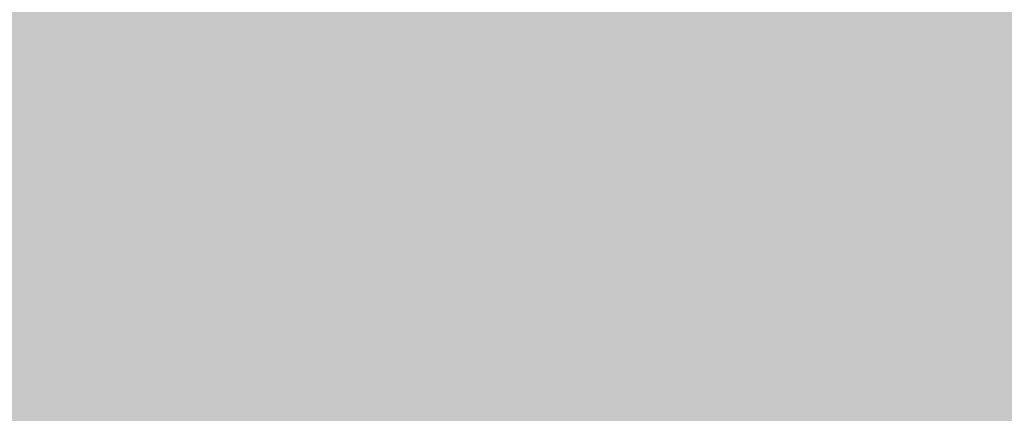
# Model space of a CAD drawing. Units: millimetres. Extents: x -22994 to 29398, y -19990 to 20176.
# Tile 100 of 135: x 229.428 to 230.597, y 84.732 to 85.199. Entities that reach past the tile are written whole.
import ezdxf
from ezdxf import colors
from ezdxf.entities.mleader import LeaderData, LeaderLine
from ezdxf.math import Vec2, Vec3

# ---------------------------------------------------------------- set-up
doc = ezdxf.new("R2010")
doc.units = ezdxf.units.MM
doc.header["$MEASUREMENT"] = 0
doc.layers.add('M-ANNO-TEXT', color=7, linetype='Continuous', lineweight=25)
doc.layers.add('M-DIMS', color=2, linetype='Continuous', lineweight=18)
doc.styles.get("Standard").update_dxf_attribs({"font": 'arial.ttf'})
doc.dimstyles.get("Standard").update_dxf_attribs({"dimtxt": 0.18, "dimasz": 10000, "dimexe": 0.18, "dimexo": 0.0625, "dimgap": 0.09, "dimtad": 0, "dimtih": 1, "dimtoh": 1, "dimdec": 0, "dimzin": 0, "dimdsep": 46, "dimtxsty": 'Standard', "dimcen": 0.09, "dimadec": 0, "dimazin": 0, "dimtfac": 1, "dimtdec": 0, "dimtofl": 0, "dimtmove": 0, "dimatfit": 3, "dimfxl": 1, "dimtolj": 1, "dimtzin": 0, "dimlwd": 30, "dimarcsym": 0})

# ---------------------------------------------------------------- blocks, each defined once
blk = doc.blocks.new('*D2')
at = {"layer": 'Defpoints', "color": 0, "transparency": 16777216}
for p in [(6.6773, 10.2713), (290.852, 10.2713), (290.852, -5.0787)]:
    blk.add_point(p, dxfattribs=at)
at = {"layer": 'M-DIMS', "color": 0, "lineweight": -2, "transparency": 16777216}
for p, q in [((6.6773, 10.2088), (6.6773, -5.2587)), ((290.852, 10.2088), (290.852, -5.2587))]:
    blk.add_line(p, q, dxfattribs=at)
at = {"layer": 'M-DIMS', "color": 0, "lineweight": 30, "transparency": 16777216}
for p, q in [((-9993.3227, -5.0787), (-19993.3227, -5.0787)), ((10290.852, -5.0787), (20290.852, -5.0787))]:
    blk.add_line(p, q, dxfattribs=at)
at = {"layer": 'M-DIMS', "color": 0, "transparency": 16777216}
for points in [[(-9993.3227, 1661.5879), (-9993.3227, -1671.7454), (6.6773, -5.0787)], [(10290.852, 1661.5879), (10290.852, -1671.7454), (290.852, -5.0787)]]:
    blk.add_solid(points, dxfattribs=at)
at = {"layer": 'M-DIMS', "color": 0, "transparency": 16777216, "insert": (148.7647, -5.0787), "char_height": 0.18, "attachment_point": 5}
blk.add_mtext('\\A1;284.2', dxfattribs=at)
blk = doc.blocks.new('*D3')
at = {"layer": 'Defpoints', "color": 0, "transparency": 16777216}
for p in [(110.2647, 204.1654), (110.2647, 176.3662), (95.8327, 127.967)]:
    blk.add_point(p, dxfattribs=at)
at = {"layer": 'M-DIMS', "color": 0, "lineweight": -2, "transparency": 16777216}
for p, q in [((95.8327, 128.0295), (95.8327, 204.3454)), ((110.2647, 176.4287), (110.2647, 204.3454))]:
    blk.add_line(p, q, dxfattribs=at)
at = {"layer": 'M-DIMS', "color": 0, "lineweight": 30, "transparency": 16777216}
for p, q in [((-9904.1673, 204.1654), (-19904.1673, 204.1654)), ((10110.2647, 204.1654), (20110.2647, 204.1654))]:
    blk.add_line(p, q, dxfattribs=at)
at = {"layer": 'M-DIMS', "color": 0, "transparency": 16777216}
for points in [[(-9904.1673, 1870.8321), (-9904.1673, -1462.5013), (95.8327, 204.1654)], [(10110.2647, 1870.8321), (10110.2647, -1462.5013), (110.2647, 204.1654)]]:
    blk.add_solid(points, dxfattribs=at)
at = {"layer": 'M-DIMS', "color": 0, "transparency": 16777216, "insert": (103.0487, 204.1654), "char_height": 0.18, "attachment_point": 5}
blk.add_mtext('\\A1;14.432', dxfattribs=at)
blk = doc.blocks.new('*D4')
at = {"layer": 'Defpoints', "color": 0, "transparency": 16777216}
for p in [(116.2647, 204.1654), (110.2647, 176.3662), (116.2647, 176.3662)]:
    blk.add_point(p, dxfattribs=at)
at = {"layer": 'M-DIMS', "color": 0, "lineweight": -2, "transparency": 16777216}
for p, q in [((110.2647, 176.4287), (110.2647, 204.3454)), ((116.2647, 176.4287), (116.2647, 204.3454))]:
    blk.add_line(p, q, dxfattribs=at)
at = {"layer": 'M-DIMS', "color": 0, "lineweight": 30, "transparency": 16777216}
for p, q in [((-9889.7353, 204.1654), (-19889.7353, 204.1654)), ((10116.2647, 204.1654), (20116.2647, 204.1654))]:
    blk.add_line(p, q, dxfattribs=at)
at = {"layer": 'M-DIMS', "color": 0, "transparency": 16777216}
for points in [[(-9889.7353, 1870.8321), (-9889.7353, -1462.5013), (110.2647, 204.1654)], [(10116.2647, 1870.8321), (10116.2647, -1462.5013), (116.2647, 204.1654)]]:
    blk.add_solid(points, dxfattribs=at)
at = {"layer": 'M-DIMS', "color": 0, "transparency": 16777216, "insert": (113.2647, 204.1654), "char_height": 0.18, "attachment_point": 5}
blk.add_mtext('\\A1;6', dxfattribs=at)
blk = doc.blocks.new('*D5')
at = {"layer": 'Defpoints', "color": 0, "transparency": 16777216}
for p in [(181.2647, 204.1654), (116.2647, 176.3662), (181.2647, 176.3662)]:
    blk.add_point(p, dxfattribs=at)
at = {"layer": 'M-DIMS', "color": 0, "lineweight": -2, "transparency": 16777216}
for p, q in [((116.2647, 176.4287), (116.2647, 204.3454)), ((181.2647, 176.4287), (181.2647, 204.3454))]:
    blk.add_line(p, q, dxfattribs=at)
at = {"layer": 'M-DIMS', "color": 0, "lineweight": 30, "transparency": 16777216}
for p, q in [((-9883.7353, 204.1654), (-19883.7353, 204.1654)), ((10181.2647, 204.1654), (20181.2647, 204.1654))]:
    blk.add_line(p, q, dxfattribs=at)
at = {"layer": 'M-DIMS', "color": 0, "transparency": 16777216}
for points in [[(-9883.7353, 1870.8321), (-9883.7353, -1462.5013), (116.2647, 204.1654)], [(10181.2647, 1870.8321), (10181.2647, -1462.5013), (181.2647, 204.1654)]]:
    blk.add_solid(points, dxfattribs=at)
at = {"layer": 'M-DIMS', "color": 0, "transparency": 16777216, "insert": (148.7647, 204.1654), "char_height": 0.18, "attachment_point": 5}
blk.add_mtext('\\A1;65', dxfattribs=at)
blk = doc.blocks.new('*D6')
at = {"layer": 'Defpoints', "color": 0, "transparency": 16777216}
for p in [(187.2647, 204.1654), (181.2647, 176.3662), (187.2647, 176.3662)]:
    blk.add_point(p, dxfattribs=at)
at = {"layer": 'M-DIMS', "color": 0, "lineweight": -2, "transparency": 16777216}
for p, q in [((181.2647, 176.4287), (181.2647, 204.3454)), ((187.2647, 176.4287), (187.2647, 204.3454))]:
    blk.add_line(p, q, dxfattribs=at)
at = {"layer": 'M-DIMS', "color": 0, "lineweight": 30, "transparency": 16777216}
for p, q in [((-9818.7353, 204.1654), (-19818.7353, 204.1654)), ((10187.2647, 204.1654), (20187.2647, 204.1654))]:
    blk.add_line(p, q, dxfattribs=at)
at = {"layer": 'M-DIMS', "color": 0, "transparency": 16777216}
for points in [[(-9818.7353, 1870.8321), (-9818.7353, -1462.5013), (181.2647, 204.1654)], [(10187.2647, 1870.8321), (10187.2647, -1462.5013), (187.2647, 204.1654)]]:
    blk.add_solid(points, dxfattribs=at)
at = {"layer": 'M-DIMS', "color": 0, "transparency": 16777216, "insert": (184.2647, 204.1654), "char_height": 0.18, "attachment_point": 5}
blk.add_mtext('\\A1;6', dxfattribs=at)
blk = doc.blocks.new('*D7')
at = {"layer": 'Defpoints', "color": 0, "transparency": 16777216}
for p in [(201.6967, 204.1654), (187.2647, 176.3662), (201.6967, 127.967)]:
    blk.add_point(p, dxfattribs=at)
at = {"layer": 'M-DIMS', "color": 0, "lineweight": -2, "transparency": 16777216}
for p, q in [((187.2647, 176.4287), (187.2647, 204.3454)), ((201.6967, 128.0295), (201.6967, 204.3454))]:
    blk.add_line(p, q, dxfattribs=at)
at = {"layer": 'M-DIMS', "color": 0, "lineweight": 30, "transparency": 16777216}
for p, q in [((-9812.7353, 204.1654), (-19812.7353, 204.1654)), ((10201.6967, 204.1654), (20201.6967, 204.1654))]:
    blk.add_line(p, q, dxfattribs=at)
at = {"layer": 'M-DIMS', "color": 0, "transparency": 16777216}
for points in [[(-9812.7353, 1870.8321), (-9812.7353, -1462.5013), (187.2647, 204.1654)], [(10201.6967, 1870.8321), (10201.6967, -1462.5013), (201.6967, 204.1654)]]:
    blk.add_solid(points, dxfattribs=at)
at = {"layer": 'M-DIMS', "color": 0, "transparency": 16777216, "insert": (194.4807, 204.1654), "char_height": 0.18, "attachment_point": 5}
blk.add_mtext('\\A1;14.432', dxfattribs=at)
blk = doc.blocks.new('*D8')
at = {"layer": 'Defpoints', "color": 0, "transparency": 16777216}
for p in [(227.6485, 204.1654), (227.6485, 146.7296), (201.6967, 127.967)]:
    blk.add_point(p, dxfattribs=at)
at = {"layer": 'M-DIMS', "color": 0, "lineweight": -2, "transparency": 16777216}
for p, q in [((201.6967, 128.0295), (201.6967, 204.3454)), ((227.6485, 146.7921), (227.6485, 204.3454))]:
    blk.add_line(p, q, dxfattribs=at)
at = {"layer": 'M-DIMS', "color": 0, "lineweight": 30, "transparency": 16777216}
for p, q in [((-9798.3033, 204.1654), (-19798.3033, 204.1654)), ((10227.6485, 204.1654), (20227.6485, 204.1654))]:
    blk.add_line(p, q, dxfattribs=at)
at = {"layer": 'M-DIMS', "color": 0, "transparency": 16777216}
for points in [[(-9798.3033, 1870.8321), (-9798.3033, -1462.5013), (201.6967, 204.1654)], [(10227.6485, 1870.8321), (10227.6485, -1462.5013), (227.6485, 204.1654)]]:
    blk.add_solid(points, dxfattribs=at)
at = {"layer": 'M-DIMS', "color": 0, "transparency": 16777216, "insert": (214.6726, 204.1654), "char_height": 0.18, "attachment_point": 5}
blk.add_mtext('\\A1;25.95', dxfattribs=at)
blk = doc.blocks.new('*D9')
at = {"layer": 'Defpoints', "color": 0, "transparency": 16777216}
for p in [(187.2647, 176.3662), (306.202, 176.3662), (290.852, 10.2713)]:
    blk.add_point(p, dxfattribs=at)
at = {"layer": 'M-DIMS', "color": 0, "lineweight": 30, "transparency": 16777216}
for p, q in [((306.202, 10176.3662), (306.202, 20176.3662)), ((306.202, -9989.7287), (306.202, -19989.7287))]:
    blk.add_line(p, q, dxfattribs=at)
at = {"layer": 'M-DIMS', "color": 0, "lineweight": -2, "transparency": 16777216}
for p, q in [((187.3272, 176.3662), (306.382, 176.3662)), ((290.9145, 10.2713), (306.382, 10.2713))]:
    blk.add_line(p, q, dxfattribs=at)
at = {"layer": 'M-DIMS', "color": 0, "transparency": 16777216}
for points in [[(-1360.4646, 10176.3662), (1972.8687, 10176.3662), (306.202, 176.3662)], [(-1360.4646, -9989.7287), (1972.8687, -9989.7287), (306.202, 10.2713)]]:
    blk.add_solid(points, dxfattribs=at)
at = {"layer": 'M-DIMS', "color": 0, "transparency": 16777216, "insert": (306.202, 93.3187), "char_height": 0.18, "attachment_point": 5}
blk.add_mtext('\\A1;166.1', dxfattribs=at)
blk = doc.blocks.new('*D10')
at = {"layer": 'Defpoints', "color": 0, "transparency": 16777216}
for p in [(125.6498, 136.0713), (133.3459, 136.0713), (133.3459, -5.0787)]:
    blk.add_point(p, dxfattribs=at)
at = {"layer": 'M-DIMS', "color": 0, "lineweight": -2, "transparency": 16777216}
for p, q in [((125.6498, 136.0088), (125.6498, -5.2587)), ((133.3459, 136.0088), (133.3459, -5.2587))]:
    blk.add_line(p, q, dxfattribs=at)
at = {"layer": 'M-DIMS', "color": 0, "lineweight": 30, "transparency": 16777216}
for p, q in [((-9874.3502, -5.0787), (-19874.3502, -5.0787)), ((10133.3459, -5.0787), (20133.3459, -5.0787))]:
    blk.add_line(p, q, dxfattribs=at)
at = {"layer": 'M-DIMS', "color": 0, "transparency": 16777216}
for points in [[(-9874.3502, 1661.5879), (-9874.3502, -1671.7454), (125.6498, -5.0787)], [(10133.3459, 1661.5879), (10133.3459, -1671.7454), (133.3459, -5.0787)]]:
    blk.add_solid(points, dxfattribs=at)
at = {"layer": 'M-DIMS', "color": 0, "transparency": 16777216, "insert": (129.4978, -5.0787), "char_height": 0.18, "attachment_point": 5}
blk.add_mtext('\\A1;7.696', dxfattribs=at)
blk = doc.blocks.new('*D11')
at = {"layer": 'Defpoints', "color": 0, "transparency": 16777216}
for p in [(133.3459, 136.0713), (135.6498, 136.0713), (135.6498, -5.0787)]:
    blk.add_point(p, dxfattribs=at)
at = {"layer": 'M-DIMS', "color": 0, "lineweight": -2, "transparency": 16777216}
for p, q in [((133.3459, 136.0088), (133.3459, -5.2587)), ((135.6498, 136.0088), (135.6498, -5.2587))]:
    blk.add_line(p, q, dxfattribs=at)
at = {"layer": 'M-DIMS', "color": 0, "lineweight": 30, "transparency": 16777216}
for p, q in [((-9866.6541, -5.0787), (-19866.6541, -5.0787)), ((10135.6498, -5.0787), (20135.6498, -5.0787))]:
    blk.add_line(p, q, dxfattribs=at)
at = {"layer": 'M-DIMS', "color": 0, "transparency": 16777216}
for points in [[(-9866.6541, 1661.5879), (-9866.6541, -1671.7454), (133.3459, -5.0787)], [(10135.6498, 1661.5879), (10135.6498, -1671.7454), (135.6498, -5.0787)]]:
    blk.add_solid(points, dxfattribs=at)
at = {"layer": 'M-DIMS', "color": 0, "transparency": 16777216, "insert": (134.4978, -5.0787), "char_height": 0.18, "attachment_point": 5}
blk.add_mtext('\\A1;2.304', dxfattribs=at)
blk = doc.blocks.new('*D12')
at = {"layer": 'Defpoints', "color": 0, "transparency": 16777216}
for p in [(135.6498, 136.0713), (145.6498, 136.0713), (145.6498, -5.0787)]:
    blk.add_point(p, dxfattribs=at)
at = {"layer": 'M-DIMS', "color": 0, "lineweight": -2, "transparency": 16777216}
for p, q in [((135.6498, 136.0088), (135.6498, -5.2587)), ((145.6498, 136.0088), (145.6498, -5.2587))]:
    blk.add_line(p, q, dxfattribs=at)
at = {"layer": 'M-DIMS', "color": 0, "lineweight": 30, "transparency": 16777216}
for p, q in [((-9864.3502, -5.0787), (-19864.3502, -5.0787)), ((10145.6498, -5.0787), (20145.6498, -5.0787))]:
    blk.add_line(p, q, dxfattribs=at)
at = {"layer": 'M-DIMS', "color": 0, "transparency": 16777216}
for points in [[(-9864.3502, 1661.5879), (-9864.3502, -1671.7454), (135.6498, -5.0787)], [(10145.6498, 1661.5879), (10145.6498, -1671.7454), (145.6498, -5.0787)]]:
    blk.add_solid(points, dxfattribs=at)
at = {"layer": 'M-DIMS', "color": 0, "transparency": 16777216, "insert": (140.6498, -5.0787), "char_height": 0.18, "attachment_point": 5}
blk.add_mtext('\\A1;10', dxfattribs=at)
blk = doc.blocks.new('*D13')
at = {"layer": 'Defpoints', "color": 0, "transparency": 16777216}
for p in [(145.6498, 136.0713), (155.6498, 136.0713), (155.6498, -5.0787)]:
    blk.add_point(p, dxfattribs=at)
at = {"layer": 'M-DIMS', "color": 0, "lineweight": -2, "transparency": 16777216}
for p, q in [((145.6498, 136.0088), (145.6498, -5.2587)), ((155.6498, 136.0088), (155.6498, -5.2587))]:
    blk.add_line(p, q, dxfattribs=at)
at = {"layer": 'M-DIMS', "color": 0, "lineweight": 30, "transparency": 16777216}
for p, q in [((-9854.3502, -5.0787), (-19854.3502, -5.0787)), ((10155.6498, -5.0787), (20155.6498, -5.0787))]:
    blk.add_line(p, q, dxfattribs=at)
at = {"layer": 'M-DIMS', "color": 0, "transparency": 16777216}
for points in [[(-9854.3502, 1661.5879), (-9854.3502, -1671.7454), (145.6498, -5.0787)], [(10155.6498, 1661.5879), (10155.6498, -1671.7454), (155.6498, -5.0787)]]:
    blk.add_solid(points, dxfattribs=at)
at = {"layer": 'M-DIMS', "color": 0, "transparency": 16777216, "insert": (150.6498, -5.0787), "char_height": 0.18, "attachment_point": 5}
blk.add_mtext('\\A1;10', dxfattribs=at)
blk = doc.blocks.new('*D14')
at = {"layer": 'Defpoints', "color": 0, "transparency": 16777216}
for p in [(155.6498, 136.0713), (165.6498, 136.0713), (165.6498, -5.0787)]:
    blk.add_point(p, dxfattribs=at)
at = {"layer": 'M-DIMS', "color": 0, "lineweight": -2, "transparency": 16777216}
for p, q in [((155.6498, 136.0088), (155.6498, -5.2587)), ((165.6498, 136.0088), (165.6498, -5.2587))]:
    blk.add_line(p, q, dxfattribs=at)
at = {"layer": 'M-DIMS', "color": 0, "lineweight": 30, "transparency": 16777216}
for p, q in [((-9844.3502, -5.0787), (-19844.3502, -5.0787)), ((10165.6498, -5.0787), (20165.6498, -5.0787))]:
    blk.add_line(p, q, dxfattribs=at)
at = {"layer": 'M-DIMS', "color": 0, "transparency": 16777216}
for points in [[(-9844.3502, 1661.5879), (-9844.3502, -1671.7454), (155.6498, -5.0787)], [(10165.6498, 1661.5879), (10165.6498, -1671.7454), (165.6498, -5.0787)]]:
    blk.add_solid(points, dxfattribs=at)
at = {"layer": 'M-DIMS', "color": 0, "transparency": 16777216, "insert": (160.6498, -5.0787), "char_height": 0.18, "attachment_point": 5}
blk.add_mtext('\\A1;10', dxfattribs=at)
blk = doc.blocks.new('*D15')
at = {"layer": 'Defpoints', "color": 0, "transparency": 16777216}
for p in [(173.3459, 154.788), (173.3459, 136.0713), (306.202, 136.0713)]:
    blk.add_point(p, dxfattribs=at)
at = {"layer": 'M-DIMS', "color": 0, "lineweight": 30, "transparency": 16777216}
for p, q in [((306.202, 10154.788), (306.202, 20154.788)), ((306.202, -9863.9287), (306.202, -19863.9287))]:
    blk.add_line(p, q, dxfattribs=at)
at = {"layer": 'M-DIMS', "color": 0, "lineweight": -2, "transparency": 16777216}
for p, q in [((173.4084, 154.788), (306.382, 154.788)), ((173.4084, 136.0713), (306.382, 136.0713))]:
    blk.add_line(p, q, dxfattribs=at)
at = {"layer": 'M-DIMS', "color": 0, "transparency": 16777216}
for points in [[(-1360.4646, 10154.788), (1972.8687, 10154.788), (306.202, 154.788)], [(-1360.4646, -9863.9287), (1972.8687, -9863.9287), (306.202, 136.0713)]]:
    blk.add_solid(points, dxfattribs=at)
at = {"layer": 'M-DIMS', "color": 0, "transparency": 16777216, "insert": (306.202, 145.4297), "char_height": 0.18, "attachment_point": 5}
blk.add_mtext('\\A1;18.717', dxfattribs=at)
blk = doc.blocks.new('*D16')
at = {"layer": 'Defpoints', "color": 0, "transparency": 16777216}
for p in [(120.1702, 204.1654), (110.4658, 48.0349), (120.1702, 48.0349)]:
    blk.add_point(p, dxfattribs=at)
at = {"layer": 'M-DIMS', "color": 0, "lineweight": -2, "transparency": 16777216}
for p, q in [((110.4658, 48.0974), (110.4658, 204.3454)), ((120.1702, 48.0974), (120.1702, 204.3454))]:
    blk.add_line(p, q, dxfattribs=at)
at = {"layer": 'M-DIMS', "color": 0, "lineweight": 30, "transparency": 16777216}
for p, q in [((-9889.5342, 204.1654), (-19889.5342, 204.1654)), ((10120.1702, 204.1654), (20120.1702, 204.1654))]:
    blk.add_line(p, q, dxfattribs=at)
at = {"layer": 'M-DIMS', "color": 0, "transparency": 16777216}
for points in [[(-9889.5342, 1870.8321), (-9889.5342, -1462.5013), (110.4658, 204.1654)], [(10120.1702, 1870.8321), (10120.1702, -1462.5013), (120.1702, 204.1654)]]:
    blk.add_solid(points, dxfattribs=at)
at = {"layer": 'M-DIMS', "color": 0, "transparency": 16777216, "insert": (115.318, 204.1654), "char_height": 0.18, "attachment_point": 5}
blk.add_mtext('\\A1;9.704', dxfattribs=at)
blk = doc.blocks.new('*D17')
at = {"layer": 'Defpoints', "color": 0, "transparency": 16777216}
for p in [(126.1702, 204.1654), (120.1702, 48.0349), (126.1702, 48.0349)]:
    blk.add_point(p, dxfattribs=at)
at = {"layer": 'M-DIMS', "color": 0, "lineweight": -2, "transparency": 16777216}
for p, q in [((120.1702, 48.0974), (120.1702, 204.3454)), ((126.1702, 48.0974), (126.1702, 204.3454))]:
    blk.add_line(p, q, dxfattribs=at)
at = {"layer": 'M-DIMS', "color": 0, "lineweight": 30, "transparency": 16777216}
for p, q in [((-9879.8298, 204.1654), (-19879.8298, 204.1654)), ((10126.1702, 204.1654), (20126.1702, 204.1654))]:
    blk.add_line(p, q, dxfattribs=at)
at = {"layer": 'M-DIMS', "color": 0, "transparency": 16777216}
for points in [[(-9879.8298, 1870.8321), (-9879.8298, -1462.5013), (120.1702, 204.1654)], [(10126.1702, 1870.8321), (10126.1702, -1462.5013), (126.1702, 204.1654)]]:
    blk.add_solid(points, dxfattribs=at)
at = {"layer": 'M-DIMS', "color": 0, "transparency": 16777216, "insert": (123.1702, 204.1654), "char_height": 0.18, "attachment_point": 5}
blk.add_mtext('\\A1;6', dxfattribs=at)
blk = doc.blocks.new('*D18')
at = {"layer": 'Defpoints', "color": 0, "transparency": 16777216}
for p in [(132.1702, 204.1654), (126.1702, 48.0349), (132.1702, 48.0349)]:
    blk.add_point(p, dxfattribs=at)
at = {"layer": 'M-DIMS', "color": 0, "lineweight": -2, "transparency": 16777216}
for p, q in [((126.1702, 48.0974), (126.1702, 204.3454)), ((132.1702, 48.0974), (132.1702, 204.3454))]:
    blk.add_line(p, q, dxfattribs=at)
at = {"layer": 'M-DIMS', "color": 0, "lineweight": 30, "transparency": 16777216}
for p, q in [((-9873.8298, 204.1654), (-19873.8298, 204.1654)), ((10132.1702, 204.1654), (20132.1702, 204.1654))]:
    blk.add_line(p, q, dxfattribs=at)
at = {"layer": 'M-DIMS', "color": 0, "transparency": 16777216}
for points in [[(-9873.8298, 1870.8321), (-9873.8298, -1462.5013), (126.1702, 204.1654)], [(10132.1702, 1870.8321), (10132.1702, -1462.5013), (132.1702, 204.1654)]]:
    blk.add_solid(points, dxfattribs=at)
at = {"layer": 'M-DIMS', "color": 0, "transparency": 16777216, "insert": (129.1702, 204.1654), "char_height": 0.18, "attachment_point": 5}
blk.add_mtext('\\A1;6', dxfattribs=at)
blk = doc.blocks.new('*D19')
at = {"layer": 'Defpoints', "color": 0, "transparency": 16777216}
for p in [(138.1702, 204.1654), (132.1702, 48.0349), (138.1702, 48.0349)]:
    blk.add_point(p, dxfattribs=at)
at = {"layer": 'M-DIMS', "color": 0, "lineweight": -2, "transparency": 16777216}
for p, q in [((132.1702, 48.0974), (132.1702, 204.3454)), ((138.1702, 48.0974), (138.1702, 204.3454))]:
    blk.add_line(p, q, dxfattribs=at)
at = {"layer": 'M-DIMS', "color": 0, "lineweight": 30, "transparency": 16777216}
for p, q in [((-9867.8298, 204.1654), (-19867.8298, 204.1654)), ((10138.1702, 204.1654), (20138.1702, 204.1654))]:
    blk.add_line(p, q, dxfattribs=at)
at = {"layer": 'M-DIMS', "color": 0, "transparency": 16777216}
for points in [[(-9867.8298, 1870.8321), (-9867.8298, -1462.5013), (132.1702, 204.1654)], [(10138.1702, 1870.8321), (10138.1702, -1462.5013), (138.1702, 204.1654)]]:
    blk.add_solid(points, dxfattribs=at)
at = {"layer": 'M-DIMS', "color": 0, "transparency": 16777216, "insert": (135.1702, 204.1654), "char_height": 0.18, "attachment_point": 5}
blk.add_mtext('\\A1;6', dxfattribs=at)
blk = doc.blocks.new('*D20')
at = {"layer": 'Defpoints', "color": 0, "transparency": 16777216}
for p in [(144.1702, 204.1654), (138.1702, 48.0349), (144.1702, 48.0349)]:
    blk.add_point(p, dxfattribs=at)
at = {"layer": 'M-DIMS', "color": 0, "lineweight": -2, "transparency": 16777216}
for p, q in [((138.1702, 48.0974), (138.1702, 204.3454)), ((144.1702, 48.0974), (144.1702, 204.3454))]:
    blk.add_line(p, q, dxfattribs=at)
at = {"layer": 'M-DIMS', "color": 0, "lineweight": 30, "transparency": 16777216}
for p, q in [((-9861.8298, 204.1654), (-19861.8298, 204.1654)), ((10144.1702, 204.1654), (20144.1702, 204.1654))]:
    blk.add_line(p, q, dxfattribs=at)
at = {"layer": 'M-DIMS', "color": 0, "transparency": 16777216}
for points in [[(-9861.8298, 1870.8321), (-9861.8298, -1462.5013), (138.1702, 204.1654)], [(10144.1702, 1870.8321), (10144.1702, -1462.5013), (144.1702, 204.1654)]]:
    blk.add_solid(points, dxfattribs=at)
at = {"layer": 'M-DIMS', "color": 0, "transparency": 16777216, "insert": (141.1702, 204.1654), "char_height": 0.18, "attachment_point": 5}
blk.add_mtext('\\A1;6', dxfattribs=at)
blk = doc.blocks.new('*D21')
at = {"layer": 'Defpoints', "color": 0, "transparency": 16777216}
for p in [(149.1157, 204.1654), (144.1702, 48.0349), (149.1157, 48.0349)]:
    blk.add_point(p, dxfattribs=at)
at = {"layer": 'M-DIMS', "color": 0, "lineweight": -2, "transparency": 16777216}
for p, q in [((144.1702, 48.0974), (144.1702, 204.3454)), ((149.1157, 48.0974), (149.1157, 204.3454))]:
    blk.add_line(p, q, dxfattribs=at)
at = {"layer": 'M-DIMS', "color": 0, "lineweight": 30, "transparency": 16777216}
for p, q in [((-9855.8298, 204.1654), (-19855.8298, 204.1654)), ((10149.1157, 204.1654), (20149.1157, 204.1654))]:
    blk.add_line(p, q, dxfattribs=at)
at = {"layer": 'M-DIMS', "color": 0, "transparency": 16777216}
for points in [[(-9855.8298, 1870.8321), (-9855.8298, -1462.5013), (144.1702, 204.1654)], [(10149.1157, 1870.8321), (10149.1157, -1462.5013), (149.1157, 204.1654)]]:
    blk.add_solid(points, dxfattribs=at)
at = {"layer": 'M-DIMS', "color": 0, "transparency": 16777216, "insert": (146.6429, 204.1654), "char_height": 0.18, "attachment_point": 5}
blk.add_mtext('\\A1;4.945', dxfattribs=at)
blk = doc.blocks.new('*D22')
at = {"layer": 'Defpoints', "color": 0, "transparency": 16777216}
for p in [(149.1157, 30.9895), (155.1157, 30.9895), (155.1157, -5.0787)]:
    blk.add_point(p, dxfattribs=at)
at = {"layer": 'M-DIMS', "color": 0, "lineweight": -2, "transparency": 16777216}
for p, q in [((149.1157, 30.927), (149.1157, -5.2587)), ((155.1157, 30.927), (155.1157, -5.2587))]:
    blk.add_line(p, q, dxfattribs=at)
at = {"layer": 'M-DIMS', "color": 0, "lineweight": 30, "transparency": 16777216}
for p, q in [((-9850.8843, -5.0787), (-19850.8843, -5.0787)), ((10155.1157, -5.0787), (20155.1157, -5.0787))]:
    blk.add_line(p, q, dxfattribs=at)
at = {"layer": 'M-DIMS', "color": 0, "transparency": 16777216}
for points in [[(-9850.8843, 1661.5879), (-9850.8843, -1671.7454), (149.1157, -5.0787)], [(10155.1157, 1661.5879), (10155.1157, -1671.7454), (155.1157, -5.0787)]]:
    blk.add_solid(points, dxfattribs=at)
at = {"layer": 'M-DIMS', "color": 0, "transparency": 16777216, "insert": (152.1157, -5.0787), "char_height": 0.18, "attachment_point": 5}
blk.add_mtext('\\A1;6', dxfattribs=at)
blk = doc.blocks.new('*D23')
at = {"layer": 'Defpoints', "color": 0, "transparency": 16777216}
for p in [(155.1157, 30.9895), (161.1157, 30.9895), (161.1157, -5.0787)]:
    blk.add_point(p, dxfattribs=at)
at = {"layer": 'M-DIMS', "color": 0, "lineweight": -2, "transparency": 16777216}
for p, q in [((155.1157, 30.927), (155.1157, -5.2587)), ((161.1157, 30.927), (161.1157, -5.2587))]:
    blk.add_line(p, q, dxfattribs=at)
at = {"layer": 'M-DIMS', "color": 0, "lineweight": 30, "transparency": 16777216}
for p, q in [((-9844.8843, -5.0787), (-19844.8843, -5.0787)), ((10161.1157, -5.0787), (20161.1157, -5.0787))]:
    blk.add_line(p, q, dxfattribs=at)
at = {"layer": 'M-DIMS', "color": 0, "transparency": 16777216}
for points in [[(-9844.8843, 1661.5879), (-9844.8843, -1671.7454), (155.1157, -5.0787)], [(10161.1157, 1661.5879), (10161.1157, -1671.7454), (161.1157, -5.0787)]]:
    blk.add_solid(points, dxfattribs=at)
at = {"layer": 'M-DIMS', "color": 0, "transparency": 16777216, "insert": (158.1157, -5.0787), "char_height": 0.18, "attachment_point": 5}
blk.add_mtext('\\A1;6', dxfattribs=at)
blk = doc.blocks.new('*D24')
at = {"layer": 'Defpoints', "color": 0, "transparency": 16777216}
for p in [(161.1157, 30.9895), (166.4387, 30.9895), (166.4387, -5.0787)]:
    blk.add_point(p, dxfattribs=at)
at = {"layer": 'M-DIMS', "color": 0, "lineweight": -2, "transparency": 16777216}
for p, q in [((161.1157, 30.927), (161.1157, -5.2587)), ((166.4387, 30.927), (166.4387, -5.2587))]:
    blk.add_line(p, q, dxfattribs=at)
at = {"layer": 'M-DIMS', "color": 0, "lineweight": 30, "transparency": 16777216}
for p, q in [((-9838.8843, -5.0787), (-19838.8843, -5.0787)), ((10166.4387, -5.0787), (20166.4387, -5.0787))]:
    blk.add_line(p, q, dxfattribs=at)
at = {"layer": 'M-DIMS', "color": 0, "transparency": 16777216}
for points in [[(-9838.8843, 1661.5879), (-9838.8843, -1671.7454), (161.1157, -5.0787)], [(10166.4387, 1661.5879), (10166.4387, -1671.7454), (166.4387, -5.0787)]]:
    blk.add_solid(points, dxfattribs=at)
at = {"layer": 'M-DIMS', "color": 0, "transparency": 16777216, "insert": (163.7772, -5.0787), "char_height": 0.18, "attachment_point": 5}
blk.add_mtext('\\A1;5.323', dxfattribs=at)
blk = doc.blocks.new('*D25')
at = {"layer": 'Defpoints', "color": 0, "transparency": 16777216}
for p in [(166.4387, 30.9895), (172.4387, 30.9895), (172.4387, -5.0787)]:
    blk.add_point(p, dxfattribs=at)
at = {"layer": 'M-DIMS', "color": 0, "lineweight": -2, "transparency": 16777216}
for p, q in [((166.4387, 30.927), (166.4387, -5.2587)), ((172.4387, 30.927), (172.4387, -5.2587))]:
    blk.add_line(p, q, dxfattribs=at)
at = {"layer": 'M-DIMS', "color": 0, "lineweight": 30, "transparency": 16777216}
for p, q in [((-9833.5613, -5.0787), (-19833.5613, -5.0787)), ((10172.4387, -5.0787), (20172.4387, -5.0787))]:
    blk.add_line(p, q, dxfattribs=at)
at = {"layer": 'M-DIMS', "color": 0, "transparency": 16777216}
for points in [[(-9833.5613, 1661.5879), (-9833.5613, -1671.7454), (166.4387, -5.0787)], [(10172.4387, 1661.5879), (10172.4387, -1671.7454), (172.4387, -5.0787)]]:
    blk.add_solid(points, dxfattribs=at)
at = {"layer": 'M-DIMS', "color": 0, "transparency": 16777216, "insert": (169.4387, -5.0787), "char_height": 0.18, "attachment_point": 5}
blk.add_mtext('\\A1;6', dxfattribs=at)
blk = doc.blocks.new('*D26')
at = {"layer": 'Defpoints', "color": 0, "transparency": 16777216}
for p in [(172.4387, 30.9895), (178.4387, 30.9895), (178.4387, -5.0787)]:
    blk.add_point(p, dxfattribs=at)
at = {"layer": 'M-DIMS', "color": 0, "lineweight": -2, "transparency": 16777216}
for p, q in [((172.4387, 30.927), (172.4387, -5.2587)), ((178.4387, 30.927), (178.4387, -5.2587))]:
    blk.add_line(p, q, dxfattribs=at)
at = {"layer": 'M-DIMS', "color": 0, "lineweight": 30, "transparency": 16777216}
for p, q in [((-9827.5613, -5.0787), (-19827.5613, -5.0787)), ((10178.4387, -5.0787), (20178.4387, -5.0787))]:
    blk.add_line(p, q, dxfattribs=at)
at = {"layer": 'M-DIMS', "color": 0, "transparency": 16777216}
for points in [[(-9827.5613, 1661.5879), (-9827.5613, -1671.7454), (172.4387, -5.0787)], [(10178.4387, 1661.5879), (10178.4387, -1671.7454), (178.4387, -5.0787)]]:
    blk.add_solid(points, dxfattribs=at)
at = {"layer": 'M-DIMS', "color": 0, "transparency": 16777216, "insert": (175.4387, -5.0787), "char_height": 0.18, "attachment_point": 5}
blk.add_mtext('\\A1;6', dxfattribs=at)
blk = doc.blocks.new('*D27')
at = {"layer": 'Defpoints', "color": 0, "transparency": 16777216}
for p in [(178.4387, 30.9895), (188.1175, 30.9895), (188.1175, -5.0787)]:
    blk.add_point(p, dxfattribs=at)
at = {"layer": 'M-DIMS', "color": 0, "lineweight": -2, "transparency": 16777216}
for p, q in [((178.4387, 30.927), (178.4387, -5.2587)), ((188.1175, 30.927), (188.1175, -5.2587))]:
    blk.add_line(p, q, dxfattribs=at)
at = {"layer": 'M-DIMS', "color": 0, "lineweight": 30, "transparency": 16777216}
for p, q in [((-9821.5613, -5.0787), (-19821.5613, -5.0787)), ((10188.1175, -5.0787), (20188.1175, -5.0787))]:
    blk.add_line(p, q, dxfattribs=at)
at = {"layer": 'M-DIMS', "color": 0, "transparency": 16777216}
for points in [[(-9821.5613, 1661.5879), (-9821.5613, -1671.7454), (178.4387, -5.0787)], [(10188.1175, 1661.5879), (10188.1175, -1671.7454), (188.1175, -5.0787)]]:
    blk.add_solid(points, dxfattribs=at)
at = {"layer": 'M-DIMS', "color": 0, "transparency": 16777216, "insert": (183.2781, -5.0787), "char_height": 0.18, "attachment_point": 5}
blk.add_mtext('\\A1;9.679', dxfattribs=at)
blk = doc.blocks.new('*D28')
at = {"layer": 'Defpoints', "color": 0, "transparency": 16777216}
for p in [(188.1175, 48.0349), (306.202, 48.0349), (188.1175, 30.9895)]:
    blk.add_point(p, dxfattribs=at)
at = {"layer": 'M-DIMS', "color": 0, "lineweight": 30, "transparency": 16777216}
for p, q in [((306.202, 10048.0349), (306.202, 20048.0349)), ((306.202, -9969.0105), (306.202, -19969.0105))]:
    blk.add_line(p, q, dxfattribs=at)
at = {"layer": 'M-DIMS', "color": 0, "lineweight": -2, "transparency": 16777216}
for p, q in [((188.18, 48.0349), (306.382, 48.0349)), ((188.18, 30.9895), (306.382, 30.9895))]:
    blk.add_line(p, q, dxfattribs=at)
at = {"layer": 'M-DIMS', "color": 0, "transparency": 16777216}
for points in [[(-1360.4646, 10048.0349), (1972.8687, 10048.0349), (306.202, 48.0349)], [(-1360.4646, -9969.0105), (1972.8687, -9969.0105), (306.202, 30.9895)]]:
    blk.add_solid(points, dxfattribs=at)
at = {"layer": 'M-DIMS', "color": 0, "transparency": 16777216, "insert": (306.202, 39.5122), "char_height": 0.18, "attachment_point": 5}
blk.add_mtext('\\A1;17.045', dxfattribs=at)
blk = doc.blocks.new('*D29')
at = {"layer": 'Defpoints', "color": 0, "transparency": 16777216}
for p in [(36.8006, 80.045), (64.0296, 80.045)]:
    blk.add_point(p, dxfattribs=at)
at = {"layer": 'M-DIMS', "color": 0, "lineweight": -2, "transparency": 16777216}
for p, q in [((50.4151, 79.955), (50.4151, 80.135)), ((50.3251, 80.045), (50.5051, 80.045))]:
    blk.add_line(p, q, dxfattribs=at)
at = {"layer": 'M-DIMS', "color": 0, "lineweight": 30, "transparency": 16777216}
blk.add_line((20064.0296, 80.0303), (10064.0296, 80.0377), dxfattribs=at)
at = {"layer": 'M-DIMS', "color": 0, "transparency": 16777216}
blk.add_solid([(10064.0309, 1746.7043), (10064.0284, -1586.629), (64.0296, 80.045)], dxfattribs=at)
at = {"layer": 'M-DIMS', "color": 0, "transparency": 16777216, "insert": (20064.5213, 80.0303), "char_height": 0.18, "attachment_point": 5}
blk.add_mtext('\\A1;∅27.23', dxfattribs=at)
blk = doc.blocks.new('*D30')
at = {"layer": 'Defpoints', "color": 0, "transparency": 16777216}
for p in [(216.3148, 146.7291), (238.9821, 146.73)]:
    blk.add_point(p, dxfattribs=at)
at = {"layer": 'M-DIMS', "color": 0, "lineweight": 30, "transparency": 16777216}
blk.add_line((20238.9821, 147.4959), (10238.9821, 147.1129), dxfattribs=at)
at = {"layer": 'M-DIMS', "color": 0, "lineweight": -2, "transparency": 16777216}
for p, q in [((227.6485, 146.6396), (227.6485, 146.8196)), ((227.5585, 146.7296), (227.7385, 146.7296))]:
    blk.add_line(p, q, dxfattribs=at)
at = {"layer": 'M-DIMS', "color": 0, "transparency": 16777216}
blk.add_solid([(10238.9183, 1813.7796), (10239.0459, -1519.5537), (238.9821, 146.73)], dxfattribs=at)
at = {"layer": 'M-DIMS', "color": 0, "transparency": 16777216, "insert": (20239.5436, 147.4959), "char_height": 0.18, "attachment_point": 5}
blk.add_mtext('\\A1;∅22.667', dxfattribs=at)
blk = doc.blocks.new('*D31')
at = {"layer": 'Defpoints', "color": 0, "transparency": 16777216}
for p in [(223.1641, 146.7291), (232.1328, 146.73)]:
    blk.add_point(p, dxfattribs=at)
at = {"layer": 'M-DIMS', "color": 0, "lineweight": 30, "transparency": 16777216}
blk.add_line((20232.1327, 148.6656), (10232.1328, 147.6978), dxfattribs=at)
at = {"layer": 'M-DIMS', "color": 0, "lineweight": -2, "transparency": 16777216}
for p, q in [((227.6485, 146.6396), (227.6485, 146.8196)), ((227.5585, 146.7296), (227.7385, 146.7296))]:
    blk.add_line(p, q, dxfattribs=at)
at = {"layer": 'M-DIMS', "color": 0, "transparency": 16777216}
blk.add_solid([(10231.9715, 1814.3645), (10232.2941, -1518.9688), (232.1328, 146.73)], dxfattribs=at)
at = {"layer": 'M-DIMS', "color": 0, "transparency": 16777216, "insert": (20232.6245, 148.6656), "char_height": 0.18, "attachment_point": 5}
blk.add_mtext('\\A1;∅8.969', dxfattribs=at)
blk = doc.blocks.new('*D33')
at = {"layer": 'Defpoints', "color": 0, "transparency": 16777216}
for p in [(229.5613, 154.3773), (232.9972, 153.3509)]:
    blk.add_point(p, dxfattribs=at)
at = {"layer": 'M-DIMS', "color": 0, "lineweight": -2, "transparency": 16777216}
for p, q in [((229.5613, 154.2873), (229.5613, 154.4673)), ((229.4713, 154.3773), (229.6513, 154.3773))]:
    blk.add_line(p, q, dxfattribs=at)
at = {"layer": 'M-DIMS', "color": 0, "lineweight": 30, "transparency": 16777216}
for p, q in [((19396.3388, -5570.8378), (9814.668, -2708.7434)), ((29396.3388, -5570.8378), (19396.3388, -5570.8378))]:
    blk.add_line(p, q, dxfattribs=at)
at = {"layer": 'M-DIMS', "color": 0, "transparency": 16777216}
blk.add_solid([(10291.6837, -1111.7983), (9337.6523, -4305.6886), (232.9972, 153.3509)], dxfattribs=at)
at = {"layer": 'M-DIMS', "color": 0, "transparency": 16777216, "insert": (29397.0125, -5570.8378), "char_height": 0.18, "attachment_point": 5}
blk.add_mtext('\\A1;6X R3.586', dxfattribs=at)
blk = doc.blocks.new('*D36')
at = {"layer": 'Defpoints', "color": 0, "transparency": 16777216}
for p in [(46.39, 31.3035), (46.3875, 26.5934)]:
    blk.add_point(p, dxfattribs=at)
at = {"layer": 'M-DIMS', "color": 0, "lineweight": 30, "transparency": 16777216}
for p, q in [((57.1499, 20031.3006), (51.77, 10031.302)), ((10057.1499, 20031.3006), (57.1499, 20031.3006))]:
    blk.add_line(p, q, dxfattribs=at)
at = {"layer": 'M-DIMS', "color": 0, "lineweight": -2, "transparency": 16777216}
for p, q in [((46.3887, 28.8585), (46.3887, 29.0385)), ((46.2987, 28.9485), (46.4787, 28.9485))]:
    blk.add_line(p, q, dxfattribs=at)
at = {"layer": 'M-DIMS', "color": 0, "transparency": 16777216}
blk.add_solid([(-1614.8965, 10032.1987), (1718.4364, 10030.4054), (46.39, 31.3035)], dxfattribs=at)
at = {"layer": 'M-DIMS', "color": 0, "transparency": 16777216, "insert": (10057.5542, 20031.3006), "char_height": 0.18, "attachment_point": 5}
blk.add_mtext('\\A1;∅4.71', dxfattribs=at)

msp = doc.modelspace()

# ---------------------------------------------------------------- dimensions: what is measured, and where the dimension line sits
at = {"layer": 'M-DIMS'}
for base, p1, p2, override, picture, middle in [((306.202, 176.3662), (290.852, 10.2713), (187.2647, 176.3662), {"dimdec": 1, "dimlfac": 1, "dimrnd": 0, "dimzin": 0, "dimdsep": 46, "dimlunit": 2}, '*D9', (306.202, 93.3187)), ((306.202, 136.0713), (173.3459, 154.788), (173.3459, 136.0713), {"dimdec": 3, "dimlfac": 1, "dimrnd": 0, "dimzin": 0, "dimdsep": 46, "dimlunit": 2}, '*D15', (306.202, 145.4297)), ((306.202, 48.0349), (188.1175, 30.9895), (188.1175, 48.0349), {"dimdec": 3, "dimlfac": 1, "dimrnd": 0, "dimzin": 0, "dimdsep": 46, "dimlunit": 2}, '*D28', (306.202, 39.5122))]:
    dim = msp.add_linear_dim(base=base, p1=p1, p2=p2, angle=90, dimstyle='Standard', override=override, dxfattribs=at)
    dim.commit()
    dim.dimension.update_dxf_attribs({"geometry": picture, "text_midpoint": middle})
for p1, p2, override, picture, middle in [((46.3875, 26.5934), (46.39, 31.3035), {"dimdec": 2, "dimlfac": 1, "dimrnd": 0, "dimzin": 0, "dimdsep": 46, "dimlunit": 2}, '*D36', (10057.5542, 20031.3006)), ((223.1641, 146.7291), (232.1328, 146.73), {"dimdec": 3, "dimlfac": 1, "dimrnd": 0, "dimzin": 0, "dimdsep": 46, "dimlunit": 2}, '*D31', (20232.1327, 148.6656)), ((216.3148, 146.7291), (238.9821, 146.73), {"dimdec": 3, "dimlfac": 1, "dimrnd": 0, "dimzin": 0, "dimdsep": 46, "dimlunit": 2}, '*D30', (20238.9821, 147.4959))]:
    dim = msp.add_diameter_dim_2p(p1=p1, p2=p2, dimstyle='Standard', override=override, dxfattribs=at)
    dim.commit()
    dim.dimension.update_dxf_attribs({"geometry": picture, "text_midpoint": middle, "dimtype": 163})
for base, p1, p2, override, picture, middle in [((110.2647, 204.1654), (95.8327, 127.967), (110.2647, 176.3662), {"dimdec": 3, "dimlfac": 1, "dimrnd": 0, "dimzin": 0, "dimdsep": 46, "dimlunit": 2}, '*D3', (103.0487, 204.1654)), ((116.2647, 204.1654), (110.2647, 176.3662), (116.2647, 176.3662), {"dimdec": 0, "dimlfac": 1, "dimrnd": 0, "dimzin": 0, "dimdsep": 46, "dimlunit": 2}, '*D4', (113.2647, 204.1654)), ((120.1702, 204.1654), (110.4658, 48.0349), (120.1702, 48.0349), {"dimdec": 3, "dimlfac": 1, "dimrnd": 0, "dimzin": 0, "dimdsep": 46, "dimlunit": 2}, '*D16', (115.318, 204.1654)), ((181.2647, 204.1654), (116.2647, 176.3662), (181.2647, 176.3662), {"dimdec": 0, "dimlfac": 1, "dimrnd": 0, "dimzin": 0, "dimdsep": 46, "dimlunit": 2}, '*D5', (148.7647, 204.1654)), ((126.1702, 204.1654), (120.1702, 48.0349), (126.1702, 48.0349), {"dimdec": 0, "dimlfac": 1, "dimrnd": 0, "dimzin": 0, "dimdsep": 46, "dimlunit": 2}, '*D17', (123.1702, 204.1654)), ((132.1702, 204.1654), (126.1702, 48.0349), (132.1702, 48.0349), {"dimdec": 0, "dimlfac": 1, "dimrnd": 0, "dimzin": 0, "dimdsep": 46, "dimlunit": 2}, '*D18', (129.1702, 204.1654)), ((138.1702, 204.1654), (132.1702, 48.0349), (138.1702, 48.0349), {"dimdec": 0, "dimlfac": 1, "dimrnd": 0, "dimzin": 0, "dimdsep": 46, "dimlunit": 2}, '*D19', (135.1702, 204.1654)), ((144.1702, 204.1654), (138.1702, 48.0349), (144.1702, 48.0349), {"dimdec": 0, "dimlfac": 1, "dimrnd": 0, "dimzin": 0, "dimdsep": 46, "dimlunit": 2}, '*D20', (141.1702, 204.1654)), ((149.11567, 204.16539), (144.17023, 48.03494), (149.11567, 48.03494), {"dimdec": 3, "dimlfac": 1, "dimrnd": 0, "dimzin": 0, "dimdsep": 46, "dimlunit": 2}, '*D21', (146.64295, 204.16539)), ((187.2647, 204.1654), (181.2647, 176.3662), (187.2647, 176.3662), {"dimdec": 0, "dimlfac": 1, "dimrnd": 0, "dimzin": 0, "dimdsep": 46, "dimlunit": 2}, '*D6', (184.2647, 204.1654)), ((201.6967, 204.1654), (187.2647, 176.3662), (201.6967, 127.967), {"dimdec": 3, "dimlfac": 1, "dimrnd": 0, "dimzin": 0, "dimdsep": 46, "dimlunit": 2}, '*D7', (194.4807, 204.1654)), ((227.6485, 204.1654), (201.6967, 127.967), (227.6485, 146.7296), {"dimdec": 2, "dimlfac": 1, "dimrnd": 0, "dimzin": 0, "dimdsep": 46, "dimlunit": 2}, '*D8', (214.6726, 204.1654)), ((290.852, -5.0787), (6.6773, 10.2713), (290.852, 10.2713), {"dimdec": 1, "dimlfac": 1, "dimrnd": 0, "dimzin": 0, "dimdsep": 46, "dimlunit": 2}, '*D2', (148.7647, -5.0787)), ((133.3459, -5.0787), (125.6498, 136.0713), (133.3459, 136.0713), {"dimdec": 3, "dimlfac": 1, "dimrnd": 0, "dimzin": 0, "dimdsep": 46, "dimlunit": 2}, '*D10', (129.4978, -5.0787)), ((135.6498, -5.0787), (133.3459, 136.0713), (135.6498, 136.0713), {"dimdec": 3, "dimlfac": 1, "dimrnd": 0, "dimzin": 0, "dimdsep": 46, "dimlunit": 2}, '*D11', (134.4978, -5.0787)), ((145.6498, -5.0787), (135.6498, 136.0713), (145.6498, 136.0713), {"dimdec": 0, "dimlfac": 1, "dimrnd": 0, "dimzin": 0, "dimdsep": 46, "dimlunit": 2}, '*D12', (140.6498, -5.0787)), ((155.6498, -5.0787), (145.6498, 136.0713), (155.6498, 136.0713), {"dimdec": 0, "dimlfac": 1, "dimrnd": 0, "dimzin": 0, "dimdsep": 46, "dimlunit": 2}, '*D13', (150.6498, -5.0787)), ((155.1157, -5.0787), (149.1157, 30.9895), (155.1157, 30.9895), {"dimdec": 0, "dimlfac": 1, "dimrnd": 0, "dimzin": 0, "dimdsep": 46, "dimlunit": 2}, '*D22', (152.1157, -5.0787)), ((161.1157, -5.0787), (155.1157, 30.9895), (161.1157, 30.9895), {"dimdec": 0, "dimlfac": 1, "dimrnd": 0, "dimzin": 0, "dimdsep": 46, "dimlunit": 2}, '*D23', (158.1157, -5.0787)), ((165.6498, -5.0787), (155.6498, 136.0713), (165.6498, 136.0713), {"dimdec": 0, "dimlfac": 1, "dimrnd": 0, "dimzin": 0, "dimdsep": 46, "dimlunit": 2}, '*D14', (160.6498, -5.0787)), ((166.4387, -5.0787), (161.1157, 30.9895), (166.4387, 30.9895), {"dimdec": 3, "dimlfac": 1, "dimrnd": 0, "dimzin": 0, "dimdsep": 46, "dimlunit": 2}, '*D24', (163.7772, -5.0787)), ((172.4387, -5.0787), (166.4387, 30.9895), (172.4387, 30.9895), {"dimdec": 0, "dimlfac": 1, "dimrnd": 0, "dimzin": 0, "dimdsep": 46, "dimlunit": 2}, '*D25', (169.4387, -5.0787)), ((178.4387, -5.0787), (172.4387, 30.9895), (178.4387, 30.9895), {"dimdec": 0, "dimlfac": 1, "dimrnd": 0, "dimzin": 0, "dimdsep": 46, "dimlunit": 2}, '*D26', (175.4387, -5.0787)), ((188.1175, -5.0787), (178.4387, 30.9895), (188.1175, 30.9895), {"dimdec": 3, "dimlfac": 1, "dimrnd": 0, "dimzin": 0, "dimdsep": 46, "dimlunit": 2}, '*D27', (183.2781, -5.0787))]:
    dim = msp.add_linear_dim(base=base, p1=p1, p2=p2, dimstyle='Standard', override=override, dxfattribs=at)
    dim.commit()
    dim.dimension.update_dxf_attribs({"geometry": picture, "text_midpoint": middle})
dim = msp.add_diameter_dim_2p(p1=(36.8006, 80.045), p2=(64.0296, 80.045), dimstyle='Standard', override={"dimdec": 2, "dimlfac": 1, "dimrnd": 0, "dimzin": 0, "dimdsep": 46, "dimlunit": 2}, dxfattribs=at)
dim.commit()
dim.dimension.update_dxf_attribs({"geometry": '*D29', "text_midpoint": (20064.0296, 80.0303)})
dim = msp.add_radius_dim(center=(229.5613, 154.3773), mpoint=(232.9972, 153.3509), text='6X <>', dimstyle='Standard', override={"dimdec": 3, "dimlfac": 1, "dimrnd": 0, "dimzin": 0, "dimdsep": 46, "dimlunit": 2}, dxfattribs=at)
dim.commit()
dim.dimension.update_dxf_attribs({"geometry": '*D33', "text_midpoint": (29397.0125, -5570.8378)})

# ---------------------------------------------------------------- leaders
at = {"layer": 'M-ANNO-TEXT'}
ml = msp.add_multileader_mtext('Standard', dxfattribs=at)
ml.set_content('combustion chamber', color=256)
ml.set_leader_properties()
ml.build(insert=Vec2(0, 0))
ml.multileader.update_dxf_attribs({"dogleg_length": 0.36, "arrow_head_size": 200})
ctx = ml.context
ctx.base_point, ctx.char_height, ctx.arrow_head_size, ctx.landing_gap_size, ctx.plane_origin = Vec3(215.7321, 57.9149), 3, 200, 0.09, Vec3(189.1175, 57.9149)
notes = []
notes.append((ctx, [(0, (1, 1, 0), (215.3721, 57.9149), (1, 0), 0.36, [(0, [(189.1175, 57.9149)], 0, [])])]))
ctx.mtext.insert, ctx.mtext.flow_direction = Vec3(215.8221, 59.4394), 5
for ctx, leaders in notes:
    for number, flags, end, landing, length, lines in leaders:
        leader = LeaderData()
        leader.index, (leader.has_last_leader_line, leader.has_dogleg_vector, leader.attachment_direction) = number, flags
        leader.last_leader_point, leader.dogleg_vector, leader.dogleg_length = Vec3(end), Vec3(landing), length
        for number, points, colour, breaks in lines:
            line = LeaderLine()
            line.index, line.vertices, line.color, line.breaks = number, Vec3.list(points), colors.encode_raw_color(colour), breaks
            leader.lines.append(line)
        ctx.leaders.append(leader)

doc.saveas('drawing.dxf')
